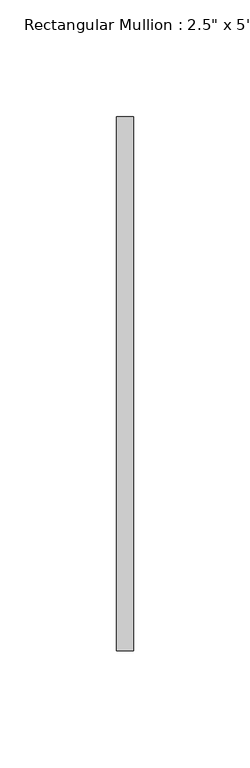
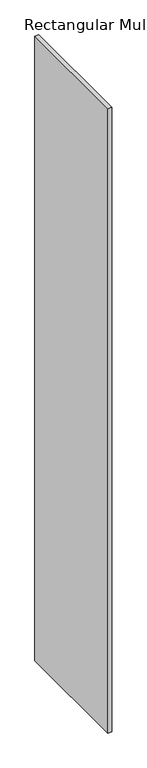
"""IFC4 building model written with IfcOpenShell, lengths in millimetres: member geometry."""

from ifc_helpers import new_model, si_unit, frame, origin, place, context, project, spatial, polyline, outline, extrude, source, transform, mapped, element, save


def member_9b8c6d2b(model_context):
    return source(origin(), model_context, "Body", "SweptSolid", [
        extrude(outline(polyline([(0.0, 114.3), (0.0, -114.3), (-7.239, -114.3), (-7.239, 114.3), (0.0, 114.3)])), frame((0.0, 0.0, -1193.8), z_axis=(0.0, 0.0, 1.0), x_axis=(1.0, 0.0, 0.0)), (0.0, 0.0, 1.0), 1193.8),
    ])


if __name__ == "__main__":
    model = new_model("IFC4")
    model_context = context("Model", 3, world=origin())
    ifc_project = project(units=[si_unit("LENGTHUNIT", "METRE", prefix="MILLI")], contexts=[model_context])
    site = spatial("IfcSite", under=ifc_project)
    building = spatial("IfcBuilding", under=site)
    placement = place(None, origin())
    member_shape = member_9b8c6d2b(model_context)
    element("IfcMember", 1, ObjectType="Rectangular Mullion : 2.5\" x 5\" rectangular", at=placement, inside=building, context=model_context, shape_type="MappedRepresentation", body=[
        mapped(member_shape, transform((0.0, 0.0, 0.0), x_axis=(1.0, 0.0, 0.0), y_axis=(0.0, 1.0, 0.0), z_axis=(0.0, 0.0, 1.0))),
    ])
    save(model, "model.ifc")

# Revit data of these elements
# Type "Rectangular Mullion : 2.5\" x 5\" rectangular"
#   built-in parameter 1007304 = 0.75 (stored number, unit not read)
#   built-in parameter 1007301 = 0.011875 (stored number, unit not read)
#   built-in parameter 1007300 = 0.011875 (stored number, unit not read)
# Element 1 (IfcMember, "Rectangular Mullion : 2.5\" x 5\" rectangular")
#   Materials on its faces: "WINDOW GLASS MATERIAL"
# Materials
#   "WINDOW GLASS MATERIAL": class "Generic", colour RGB 120 120 120, transparency 0, Cost = 0
